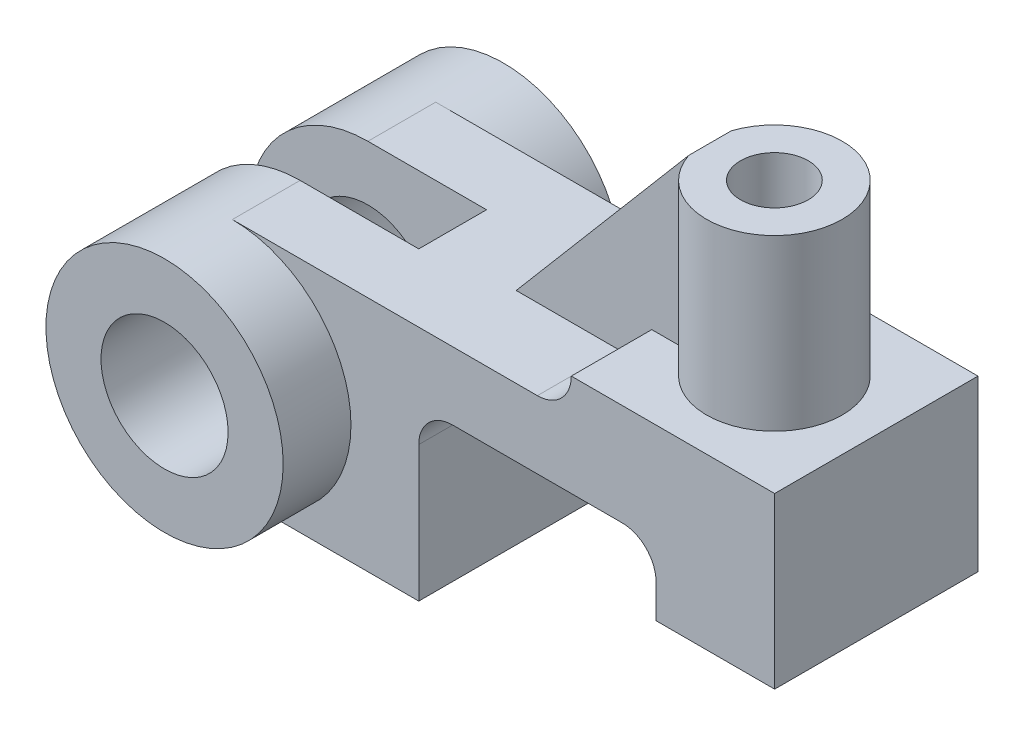
ISO-10303-21;
HEADER;
FILE_DESCRIPTION(('STEP AP214'),'2;1');
FILE_NAME('part.step','',(''),(''),'','','');
FILE_SCHEMA(('AUTOMOTIVE_DESIGN { 1 0 10303 214 1 1 1 1 }'));
ENDSEC;
DATA;
#1=APPLICATION_CONTEXT('core data for automotive mechanical design processes');
#2=APPLICATION_PROTOCOL_DEFINITION('international standard','automotive_design',2000,#1);
#3=PRODUCT_CONTEXT('',#1,'mechanical');
#4=PRODUCT('Part','Part','',(#3));
#5=PRODUCT_RELATED_PRODUCT_CATEGORY('part','',(#4));
#6=PRODUCT_DEFINITION_FORMATION('','',#4);
#7=PRODUCT_DEFINITION_CONTEXT('part definition',#1,'design');
#8=PRODUCT_DEFINITION('design','',#6,#7);
#9=PRODUCT_DEFINITION_SHAPE('','',#8);
#10=(LENGTH_UNIT() NAMED_UNIT(*) SI_UNIT(.MILLI.,.METRE.));
#11=(NAMED_UNIT(*) PLANE_ANGLE_UNIT() SI_UNIT($,.RADIAN.));
#12=(NAMED_UNIT(*) SI_UNIT($,.STERADIAN.) SOLID_ANGLE_UNIT());
#13=UNCERTAINTY_MEASURE_WITH_UNIT(LENGTH_MEASURE(1.E-05),#10,'distance_accuracy_value','');
#14=(GEOMETRIC_REPRESENTATION_CONTEXT(3) GLOBAL_UNCERTAINTY_ASSIGNED_CONTEXT((#13)) GLOBAL_UNIT_ASSIGNED_CONTEXT((#10,
#11,#12)) REPRESENTATION_CONTEXT('',''));
#15=CARTESIAN_POINT('',(0.,0.,0.));
#16=DIRECTION('',(0.,0.,1.));
#17=DIRECTION('',(1.,0.,0.));
#18=AXIS2_PLACEMENT_3D('',#15,#16,#17);
#19=CARTESIAN_POINT('',(72.,36.,24.));
#20=DIRECTION('',(0.,0.,-1.));
#21=DIRECTION('',(-1.,0.,0.));
#22=AXIS2_PLACEMENT_3D('',#19,#20,#21);
#23=CYLINDRICAL_SURFACE('',#22,8.00000000000003);
#24=DIRECTION('',(0.,0.,-1.));
#25=VECTOR('',#24,1.);
#26=CARTESIAN_POINT('',(72.,28.,24.));
#27=LINE('',#26,#25);
#28=CARTESIAN_POINT('',(72.,28.,-5.));
#29=VERTEX_POINT('',#28);
#30=CARTESIAN_POINT('',(72.,28.,-24.));
#31=VERTEX_POINT('',#30);
#32=EDGE_CURVE('E313',#29,#31,#27,.T.);
#33=ORIENTED_EDGE('',*,*,#32,.F.);
#34=CARTESIAN_POINT('',(72.,36.,-5.));
#35=DIRECTION('',(0.,0.,-1.));
#36=DIRECTION('',(-1.,0.,0.));
#37=AXIS2_PLACEMENT_3D('',#34,#35,#36);
#38=CIRCLE('',#37,8.00000000000003);
#39=CARTESIAN_POINT('',(80.,36.,-5.));
#40=VERTEX_POINT('',#39);
#41=EDGE_CURVE('E521',#40,#29,#38,.T.);
#42=ORIENTED_EDGE('',*,*,#41,.F.);
#43=DIRECTION('',(0.,0.,-1.));
#44=VECTOR('',#43,1.);
#45=CARTESIAN_POINT('',(80.,36.,24.));
#46=LINE('',#45,#44);
#47=CARTESIAN_POINT('',(80.,36.,-24.));
#48=VERTEX_POINT('',#47);
#49=EDGE_CURVE('E312',#40,#48,#46,.T.);
#50=ORIENTED_EDGE('',*,*,#49,.T.);
#51=CARTESIAN_POINT('',(72.,36.,-24.));
#52=DIRECTION('',(0.,0.,-1.));
#53=DIRECTION('',(1.,0.,0.));
#54=AXIS2_PLACEMENT_3D('',#51,#52,#53);
#55=CIRCLE('',#54,8.00000000000003);
#56=EDGE_CURVE('E304',#48,#31,#55,.T.);
#57=ORIENTED_EDGE('',*,*,#56,.T.);
#58=EDGE_LOOP('',(#33,#42,#50,#57));
#59=FACE_BOUND('',#58,.T.);
#60=ADVANCED_FACE('F44',(#59),#23,.F.);
#61=CARTESIAN_POINT('',(0.,0.,40.));
#62=DIRECTION('',(0.,0.,-1.));
#63=DIRECTION('',(-1.,0.,0.));
#64=AXIS2_PLACEMENT_3D('',#61,#62,#63);
#65=CYLINDRICAL_SURFACE('',#64,28.);
#66=CARTESIAN_POINT('',(0.,0.,-40.));
#67=DIRECTION('',(0.,0.,1.));
#68=DIRECTION('',(1.,0.,0.));
#69=AXIS2_PLACEMENT_3D('',#66,#67,#68);
#70=CIRCLE('',#69,28.);
#71=CARTESIAN_POINT('',(28.,0.,-40.));
#72=VERTEX_POINT('',#71);
#73=EDGE_CURVE('E349',#72,#72,#70,.T.);
#74=ORIENTED_EDGE('',*,*,#73,.T.);
#75=EDGE_LOOP('',(#74));
#76=FACE_BOUND('',#75,.T.);
#77=DIRECTION('',(0.,0.,-1.));
#78=VECTOR('',#77,1.);
#79=CARTESIAN_POINT('',(0.,-28.,24.));
#80=LINE('',#79,#78);
#81=CARTESIAN_POINT('',(0.,-28.,-8.));
#82=VERTEX_POINT('',#81);
#83=CARTESIAN_POINT('',(0.,-28.,-24.));
#84=VERTEX_POINT('',#83);
#85=EDGE_CURVE('E344',#82,#84,#80,.T.);
#86=ORIENTED_EDGE('',*,*,#85,.F.);
#87=CARTESIAN_POINT('',(0.,0.,-8.));
#88=DIRECTION('',(0.,0.,-1.));
#89=DIRECTION('',(-1.,0.,0.));
#90=AXIS2_PLACEMENT_3D('',#87,#88,#89);
#91=CIRCLE('',#90,28.);
#92=CARTESIAN_POINT('',(0.,28.,-8.));
#93=VERTEX_POINT('',#92);
#94=EDGE_CURVE('E250',#82,#93,#91,.T.);
#95=ORIENTED_EDGE('',*,*,#94,.T.);
#96=DIRECTION('',(0.,0.,-1.));
#97=VECTOR('',#96,1.);
#98=CARTESIAN_POINT('',(0.,28.,24.));
#99=LINE('',#98,#97);
#100=CARTESIAN_POINT('',(0.,28.,-24.));
#101=VERTEX_POINT('',#100);
#102=EDGE_CURVE('E282',#93,#101,#99,.T.);
#103=ORIENTED_EDGE('',*,*,#102,.T.);
#104=CARTESIAN_POINT('',(0.,0.,-24.));
#105=DIRECTION('',(0.,0.,-1.));
#106=DIRECTION('',(1.,0.,0.));
#107=AXIS2_PLACEMENT_3D('',#104,#105,#106);
#108=CIRCLE('',#107,28.);
#109=EDGE_CURVE('E251',#101,#84,#108,.T.);
#110=ORIENTED_EDGE('',*,*,#109,.T.);
#111=EDGE_LOOP('',(#86,#95,#103,#110));
#112=FACE_BOUND('',#111,.T.);
#113=ADVANCED_FACE('F404',(#76,#112),#65,.T.);
#114=CARTESIAN_POINT('',(0.,0.,40.));
#115=DIRECTION('',(0.,0.,-1.));
#116=DIRECTION('',(-1.,0.,0.));
#117=AXIS2_PLACEMENT_3D('',#114,#115,#116);
#118=CYLINDRICAL_SURFACE('',#117,15.);
#119=CARTESIAN_POINT('',(0.,0.,-8.));
#120=DIRECTION('',(0.,0.,-1.));
#121=DIRECTION('',(-1.,0.,0.));
#122=AXIS2_PLACEMENT_3D('',#119,#120,#121);
#123=CIRCLE('',#122,15.);
#124=CARTESIAN_POINT('',(-15.,0.,-8.));
#125=VERTEX_POINT('',#124);
#126=EDGE_CURVE('E247',#125,#125,#123,.T.);
#127=ORIENTED_EDGE('',*,*,#126,.F.);
#128=EDGE_LOOP('',(#127));
#129=FACE_BOUND('',#128,.T.);
#130=CARTESIAN_POINT('',(0.,0.,-40.));
#131=DIRECTION('',(0.,0.,1.));
#132=DIRECTION('',(1.,0.,0.));
#133=AXIS2_PLACEMENT_3D('',#130,#131,#132);
#134=CIRCLE('',#133,15.);
#135=CARTESIAN_POINT('',(15.,0.,-40.));
#136=VERTEX_POINT('',#135);
#137=EDGE_CURVE('E345',#136,#136,#134,.T.);
#138=ORIENTED_EDGE('',*,*,#137,.F.);
#139=EDGE_LOOP('',(#138));
#140=FACE_BOUND('',#139,.T.);
#141=ADVANCED_FACE('F411',(#129,#140),#118,.F.);
#142=CARTESIAN_POINT('',(0.,0.,40.));
#143=DIRECTION('',(0.,0.,1.));
#144=DIRECTION('',(1.,0.,0.));
#145=AXIS2_PLACEMENT_3D('',#142,#143,#144);
#146=PLANE('',#145);
#147=CARTESIAN_POINT('',(0.,0.,40.));
#148=DIRECTION('',(0.,0.,1.));
#149=DIRECTION('',(1.,0.,0.));
#150=AXIS2_PLACEMENT_3D('',#147,#148,#149);
#151=CIRCLE('',#150,28.);
#152=CARTESIAN_POINT('',(28.,0.,40.));
#153=VERTEX_POINT('',#152);
#154=EDGE_CURVE('E355',#153,#153,#151,.T.);
#155=ORIENTED_EDGE('',*,*,#154,.T.);
#156=EDGE_LOOP('',(#155));
#157=FACE_BOUND('',#156,.T.);
#158=CARTESIAN_POINT('',(0.,0.,40.));
#159=DIRECTION('',(0.,0.,1.));
#160=DIRECTION('',(1.,0.,0.));
#161=AXIS2_PLACEMENT_3D('',#158,#159,#160);
#162=CIRCLE('',#161,15.);
#163=CARTESIAN_POINT('',(15.,0.,40.));
#164=VERTEX_POINT('',#163);
#165=EDGE_CURVE('E347',#164,#164,#162,.T.);
#166=ORIENTED_EDGE('',*,*,#165,.F.);
#167=EDGE_LOOP('',(#166));
#168=FACE_BOUND('',#167,.T.);
#169=ADVANCED_FACE('F458',(#157,#168),#146,.T.);
#170=CARTESIAN_POINT('',(0.,0.,-40.));
#171=DIRECTION('',(0.,0.,1.));
#172=DIRECTION('',(1.,0.,0.));
#173=AXIS2_PLACEMENT_3D('',#170,#171,#172);
#174=PLANE('',#173);
#175=ORIENTED_EDGE('',*,*,#73,.F.);
#176=EDGE_LOOP('',(#175));
#177=FACE_BOUND('',#176,.T.);
#178=ORIENTED_EDGE('',*,*,#137,.T.);
#179=EDGE_LOOP('',(#178));
#180=FACE_BOUND('',#179,.T.);
#181=ADVANCED_FACE('F465',(#177,#180),#174,.F.);
#182=CARTESIAN_POINT('',(0.,28.,24.));
#183=VERTEX_POINT('',#182);
#184=CARTESIAN_POINT('',(0.,28.,8.));
#185=VERTEX_POINT('',#184);
#186=EDGE_CURVE('E306',#183,#185,#99,.T.);
#187=ORIENTED_EDGE('',*,*,#186,.T.);
#188=CARTESIAN_POINT('',(0.,0.,8.));
#189=DIRECTION('',(0.,0.,1.));
#190=DIRECTION('',(1.,0.,0.));
#191=AXIS2_PLACEMENT_3D('',#188,#189,#190);
#192=CIRCLE('',#191,28.);
#193=CARTESIAN_POINT('',(0.,-28.,8.));
#194=VERTEX_POINT('',#193);
#195=EDGE_CURVE('E58',#185,#194,#192,.T.);
#196=ORIENTED_EDGE('',*,*,#195,.T.);
#197=CARTESIAN_POINT('',(0.,-28.,24.));
#198=VERTEX_POINT('',#197);
#199=EDGE_CURVE('E67',#198,#194,#80,.T.);
#200=ORIENTED_EDGE('',*,*,#199,.F.);
#201=CARTESIAN_POINT('',(0.,0.,24.));
#202=DIRECTION('',(0.,0.,-1.));
#203=DIRECTION('',(1.,0.,0.));
#204=AXIS2_PLACEMENT_3D('',#201,#202,#203);
#205=CIRCLE('',#204,28.);
#206=EDGE_CURVE('E255',#183,#198,#205,.T.);
#207=ORIENTED_EDGE('',*,*,#206,.F.);
#208=EDGE_LOOP('',(#187,#196,#200,#207));
#209=FACE_BOUND('',#208,.T.);
#210=ORIENTED_EDGE('',*,*,#154,.F.);
#211=EDGE_LOOP('',(#210));
#212=FACE_BOUND('',#211,.T.);
#213=ADVANCED_FACE('F50',(#209,#212),#65,.T.);
#214=CARTESIAN_POINT('',(0.,0.,8.));
#215=DIRECTION('',(0.,0.,1.));
#216=DIRECTION('',(1.,0.,0.));
#217=AXIS2_PLACEMENT_3D('',#214,#215,#216);
#218=CIRCLE('',#217,15.);
#219=CARTESIAN_POINT('',(15.,0.,8.));
#220=VERTEX_POINT('',#219);
#221=EDGE_CURVE('E242',#220,#220,#218,.T.);
#222=ORIENTED_EDGE('',*,*,#221,.F.);
#223=EDGE_LOOP('',(#222));
#224=FACE_BOUND('',#223,.T.);
#225=ORIENTED_EDGE('',*,*,#165,.T.);
#226=EDGE_LOOP('',(#225));
#227=FACE_BOUND('',#226,.T.);
#228=ADVANCED_FACE('F455',(#224,#227),#118,.F.);
#229=CARTESIAN_POINT('',(44.,-28.,24.));
#230=DIRECTION('',(0.,1.,0.));
#231=DIRECTION('',(-1.,0.,0.));
#232=AXIS2_PLACEMENT_3D('',#229,#230,#231);
#233=PLANE('',#232);
#234=DIRECTION('',(0.,0.,-1.));
#235=VECTOR('',#234,1.);
#236=CARTESIAN_POINT('',(28.,-28.,-8.));
#237=LINE('',#236,#235);
#238=CARTESIAN_POINT('',(28.,-28.,8.));
#239=VERTEX_POINT('',#238);
#240=CARTESIAN_POINT('',(28.,-28.,-8.));
#241=VERTEX_POINT('',#240);
#242=EDGE_CURVE('E231',#239,#241,#237,.T.);
#243=ORIENTED_EDGE('',*,*,#242,.T.);
#244=DIRECTION('',(-1.,0.,0.));
#245=VECTOR('',#244,1.);
#246=CARTESIAN_POINT('',(-35.2475217836103,-28.,-8.));
#247=LINE('',#246,#245);
#248=EDGE_CURVE('E233',#241,#82,#247,.T.);
#249=ORIENTED_EDGE('',*,*,#248,.T.);
#250=ORIENTED_EDGE('',*,*,#85,.T.);
#251=DIRECTION('',(1.,0.,0.));
#252=VECTOR('',#251,1.);
#253=CARTESIAN_POINT('',(44.,-28.,-24.));
#254=LINE('',#253,#252);
#255=CARTESIAN_POINT('',(44.,-28.,-24.));
#256=VERTEX_POINT('',#255);
#257=EDGE_CURVE('E284',#84,#256,#254,.T.);
#258=ORIENTED_EDGE('',*,*,#257,.T.);
#259=DIRECTION('',(0.,0.,-1.));
#260=VECTOR('',#259,1.);
#261=CARTESIAN_POINT('',(44.,-28.,24.));
#262=LINE('',#261,#260);
#263=CARTESIAN_POINT('',(44.,-28.,24.));
#264=VERTEX_POINT('',#263);
#265=EDGE_CURVE('E336',#264,#256,#262,.T.);
#266=ORIENTED_EDGE('',*,*,#265,.F.);
#267=DIRECTION('',(1.,0.,0.));
#268=VECTOR('',#267,1.);
#269=CARTESIAN_POINT('',(44.,-28.,24.));
#270=LINE('',#269,#268);
#271=EDGE_CURVE('E260',#198,#264,#270,.T.);
#272=ORIENTED_EDGE('',*,*,#271,.F.);
#273=ORIENTED_EDGE('',*,*,#199,.T.);
#274=DIRECTION('',(1.,0.,0.));
#275=VECTOR('',#274,1.);
#276=CARTESIAN_POINT('',(-35.2475217836103,-28.,8.));
#277=LINE('',#276,#275);
#278=EDGE_CURVE('E228',#194,#239,#277,.T.);
#279=ORIENTED_EDGE('',*,*,#278,.T.);
#280=EDGE_LOOP('',(#243,#249,#250,#258,#266,#272,#273,#279));
#281=FACE_BOUND('',#280,.T.);
#282=ADVANCED_FACE('F451',(#281),#233,.F.);
#283=CARTESIAN_POINT('',(44.,3.99999999999999,24.));
#284=DIRECTION('',(-1.,0.,0.));
#285=DIRECTION('',(0.,0.,1.));
#286=AXIS2_PLACEMENT_3D('',#283,#284,#285);
#287=PLANE('',#286);
#288=DIRECTION('',(0.,1.,0.));
#289=VECTOR('',#288,1.);
#290=CARTESIAN_POINT('',(44.,3.99999999999999,-24.));
#291=LINE('',#290,#289);
#292=CARTESIAN_POINT('',(44.,4.,-24.));
#293=VERTEX_POINT('',#292);
#294=EDGE_CURVE('E286',#256,#293,#291,.T.);
#295=ORIENTED_EDGE('',*,*,#294,.T.);
#296=DIRECTION('',(0.,0.,-1.));
#297=VECTOR('',#296,1.);
#298=CARTESIAN_POINT('',(44.,4.,24.));
#299=LINE('',#298,#297);
#300=CARTESIAN_POINT('',(44.,4.,24.));
#301=VERTEX_POINT('',#300);
#302=EDGE_CURVE('E340',#301,#293,#299,.T.);
#303=ORIENTED_EDGE('',*,*,#302,.F.);
#304=DIRECTION('',(0.,1.,0.));
#305=VECTOR('',#304,1.);
#306=CARTESIAN_POINT('',(44.,3.99999999999999,24.));
#307=LINE('',#306,#305);
#308=EDGE_CURVE('E257',#264,#301,#307,.T.);
#309=ORIENTED_EDGE('',*,*,#308,.F.);
#310=ORIENTED_EDGE('',*,*,#265,.T.);
#311=EDGE_LOOP('',(#295,#303,#309,#310));
#312=FACE_BOUND('',#311,.T.);
#313=ADVANCED_FACE('F450',(#312),#287,.F.);
#314=CARTESIAN_POINT('',(52.,3.99999999999999,24.));
#315=DIRECTION('',(0.,0.,-1.));
#316=DIRECTION('',(-1.,0.,0.));
#317=AXIS2_PLACEMENT_3D('',#314,#315,#316);
#318=CYLINDRICAL_SURFACE('',#317,8.);
#319=CARTESIAN_POINT('',(52.,3.99999999999999,-24.));
#320=DIRECTION('',(0.,0.,-1.));
#321=DIRECTION('',(1.,0.,0.));
#322=AXIS2_PLACEMENT_3D('',#319,#320,#321);
#323=CIRCLE('',#322,8.);
#324=CARTESIAN_POINT('',(52.,12.,-24.));
#325=VERTEX_POINT('',#324);
#326=EDGE_CURVE('E289',#293,#325,#323,.T.);
#327=ORIENTED_EDGE('',*,*,#326,.T.);
#328=DIRECTION('',(0.,0.,-1.));
#329=VECTOR('',#328,1.);
#330=CARTESIAN_POINT('',(52.,12.,24.));
#331=LINE('',#330,#329);
#332=CARTESIAN_POINT('',(52.,12.,24.));
#333=VERTEX_POINT('',#332);
#334=EDGE_CURVE('E331',#333,#325,#331,.T.);
#335=ORIENTED_EDGE('',*,*,#334,.F.);
#336=CARTESIAN_POINT('',(52.,3.99999999999999,24.));
#337=DIRECTION('',(0.,0.,-1.));
#338=DIRECTION('',(1.,0.,0.));
#339=AXIS2_PLACEMENT_3D('',#336,#337,#338);
#340=CIRCLE('',#339,8.);
#341=EDGE_CURVE('E265',#301,#333,#340,.T.);
#342=ORIENTED_EDGE('',*,*,#341,.F.);
#343=ORIENTED_EDGE('',*,*,#302,.T.);
#344=EDGE_LOOP('',(#327,#335,#342,#343));
#345=FACE_BOUND('',#344,.T.);
#346=ADVANCED_FACE('F444',(#345),#318,.F.);
#347=CARTESIAN_POINT('',(92.,12.,24.));
#348=DIRECTION('',(0.,1.,0.));
#349=DIRECTION('',(-1.,0.,0.));
#350=AXIS2_PLACEMENT_3D('',#347,#348,#349);
#351=PLANE('',#350);
#352=DIRECTION('',(1.,0.,0.));
#353=VECTOR('',#352,1.);
#354=CARTESIAN_POINT('',(92.,12.,-24.));
#355=LINE('',#354,#353);
#356=CARTESIAN_POINT('',(92.,12.,-24.));
#357=VERTEX_POINT('',#356);
#358=EDGE_CURVE('E290',#325,#357,#355,.T.);
#359=ORIENTED_EDGE('',*,*,#358,.T.);
#360=DIRECTION('',(0.,0.,-1.));
#361=VECTOR('',#360,1.);
#362=CARTESIAN_POINT('',(92.,12.,24.));
#363=LINE('',#362,#361);
#364=CARTESIAN_POINT('',(92.,12.,24.));
#365=VERTEX_POINT('',#364);
#366=EDGE_CURVE('E332',#365,#357,#363,.T.);
#367=ORIENTED_EDGE('',*,*,#366,.F.);
#368=DIRECTION('',(1.,0.,0.));
#369=VECTOR('',#368,1.);
#370=CARTESIAN_POINT('',(92.,12.,24.));
#371=LINE('',#370,#369);
#372=EDGE_CURVE('E262',#333,#365,#371,.T.);
#373=ORIENTED_EDGE('',*,*,#372,.F.);
#374=ORIENTED_EDGE('',*,*,#334,.T.);
#375=EDGE_LOOP('',(#359,#367,#373,#374));
#376=FACE_BOUND('',#375,.T.);
#377=ADVANCED_FACE('F438',(#376),#351,.F.);
#378=CARTESIAN_POINT('',(92.,4.,24.));
#379=DIRECTION('',(0.,0.,-1.));
#380=DIRECTION('',(-1.,0.,0.));
#381=AXIS2_PLACEMENT_3D('',#378,#379,#380);
#382=CYLINDRICAL_SURFACE('',#381,8.);
#383=CARTESIAN_POINT('',(92.,4.,-24.));
#384=DIRECTION('',(0.,0.,-1.));
#385=DIRECTION('',(1.,0.,0.));
#386=AXIS2_PLACEMENT_3D('',#383,#384,#385);
#387=CIRCLE('',#386,8.);
#388=CARTESIAN_POINT('',(100.,4.,-24.));
#389=VERTEX_POINT('',#388);
#390=EDGE_CURVE('E295',#357,#389,#387,.T.);
#391=ORIENTED_EDGE('',*,*,#390,.T.);
#392=DIRECTION('',(0.,0.,-1.));
#393=VECTOR('',#392,1.);
#394=CARTESIAN_POINT('',(100.,4.,24.));
#395=LINE('',#394,#393);
#396=CARTESIAN_POINT('',(100.,4.,24.));
#397=VERTEX_POINT('',#396);
#398=EDGE_CURVE('E327',#397,#389,#395,.T.);
#399=ORIENTED_EDGE('',*,*,#398,.F.);
#400=CARTESIAN_POINT('',(92.,4.,24.));
#401=DIRECTION('',(0.,0.,-1.));
#402=DIRECTION('',(1.,0.,0.));
#403=AXIS2_PLACEMENT_3D('',#400,#401,#402);
#404=CIRCLE('',#403,8.);
#405=EDGE_CURVE('E266',#365,#397,#404,.T.);
#406=ORIENTED_EDGE('',*,*,#405,.F.);
#407=ORIENTED_EDGE('',*,*,#366,.T.);
#408=EDGE_LOOP('',(#391,#399,#406,#407));
#409=FACE_BOUND('',#408,.T.);
#410=ADVANCED_FACE('F434',(#409),#382,.F.);
#411=CARTESIAN_POINT('',(100.,-3.99999999999999,24.));
#412=DIRECTION('',(1.,0.,0.));
#413=DIRECTION('',(0.,0.,-1.));
#414=AXIS2_PLACEMENT_3D('',#411,#412,#413);
#415=PLANE('',#414);
#416=DIRECTION('',(0.,-1.,0.));
#417=VECTOR('',#416,1.);
#418=CARTESIAN_POINT('',(100.,-3.99999999999999,-24.));
#419=LINE('',#418,#417);
#420=CARTESIAN_POINT('',(100.,-3.99999999999999,-24.));
#421=VERTEX_POINT('',#420);
#422=EDGE_CURVE('E294',#389,#421,#419,.T.);
#423=ORIENTED_EDGE('',*,*,#422,.T.);
#424=DIRECTION('',(0.,0.,-1.));
#425=VECTOR('',#424,1.);
#426=CARTESIAN_POINT('',(100.,-3.99999999999999,24.));
#427=LINE('',#426,#425);
#428=CARTESIAN_POINT('',(100.,-3.99999999999999,24.));
#429=VERTEX_POINT('',#428);
#430=EDGE_CURVE('E324',#429,#421,#427,.T.);
#431=ORIENTED_EDGE('',*,*,#430,.F.);
#432=DIRECTION('',(0.,-1.,0.));
#433=VECTOR('',#432,1.);
#434=CARTESIAN_POINT('',(100.,-3.99999999999999,24.));
#435=LINE('',#434,#433);
#436=EDGE_CURVE('E268',#397,#429,#435,.T.);
#437=ORIENTED_EDGE('',*,*,#436,.F.);
#438=ORIENTED_EDGE('',*,*,#398,.T.);
#439=EDGE_LOOP('',(#423,#431,#437,#438));
#440=FACE_BOUND('',#439,.T.);
#441=ADVANCED_FACE('F431',(#440),#415,.F.);
#442=CARTESIAN_POINT('',(128.,-3.99999999999998,24.));
#443=DIRECTION('',(0.,1.,0.));
#444=DIRECTION('',(-1.,0.,0.));
#445=AXIS2_PLACEMENT_3D('',#442,#443,#444);
#446=PLANE('',#445);
#447=DIRECTION('',(1.,0.,0.));
#448=VECTOR('',#447,1.);
#449=CARTESIAN_POINT('',(128.,-3.99999999999998,-24.));
#450=LINE('',#449,#448);
#451=CARTESIAN_POINT('',(128.,-3.99999999999998,-24.));
#452=VERTEX_POINT('',#451);
#453=EDGE_CURVE('E297',#421,#452,#450,.T.);
#454=ORIENTED_EDGE('',*,*,#453,.T.);
#455=DIRECTION('',(0.,0.,-1.));
#456=VECTOR('',#455,1.);
#457=CARTESIAN_POINT('',(128.,-3.99999999999998,24.));
#458=LINE('',#457,#456);
#459=CARTESIAN_POINT('',(128.,-3.99999999999998,24.));
#460=VERTEX_POINT('',#459);
#461=EDGE_CURVE('E325',#460,#452,#458,.T.);
#462=ORIENTED_EDGE('',*,*,#461,.F.);
#463=DIRECTION('',(1.,0.,0.));
#464=VECTOR('',#463,1.);
#465=CARTESIAN_POINT('',(128.,-3.99999999999998,24.));
#466=LINE('',#465,#464);
#467=EDGE_CURVE('E269',#429,#460,#466,.T.);
#468=ORIENTED_EDGE('',*,*,#467,.F.);
#469=ORIENTED_EDGE('',*,*,#430,.T.);
#470=EDGE_LOOP('',(#454,#462,#468,#469));
#471=FACE_BOUND('',#470,.T.);
#472=ADVANCED_FACE('F424',(#471),#446,.F.);
#473=CARTESIAN_POINT('',(128.,36.,24.));
#474=DIRECTION('',(-1.,0.,0.));
#475=DIRECTION('',(0.,0.,1.));
#476=AXIS2_PLACEMENT_3D('',#473,#474,#475);
#477=PLANE('',#476);
#478=DIRECTION('',(0.,1.,0.));
#479=VECTOR('',#478,1.);
#480=CARTESIAN_POINT('',(128.,36.,-24.));
#481=LINE('',#480,#479);
#482=CARTESIAN_POINT('',(128.,36.,-24.));
#483=VERTEX_POINT('',#482);
#484=EDGE_CURVE('E298',#452,#483,#481,.T.);
#485=ORIENTED_EDGE('',*,*,#484,.T.);
#486=DIRECTION('',(0.,0.,-1.));
#487=VECTOR('',#486,1.);
#488=CARTESIAN_POINT('',(128.,36.,24.));
#489=LINE('',#488,#487);
#490=CARTESIAN_POINT('',(128.,36.,24.));
#491=VERTEX_POINT('',#490);
#492=EDGE_CURVE('E317',#491,#483,#489,.T.);
#493=ORIENTED_EDGE('',*,*,#492,.F.);
#494=DIRECTION('',(0.,1.,0.));
#495=VECTOR('',#494,1.);
#496=CARTESIAN_POINT('',(128.,36.,24.));
#497=LINE('',#496,#495);
#498=EDGE_CURVE('E275',#460,#491,#497,.T.);
#499=ORIENTED_EDGE('',*,*,#498,.F.);
#500=ORIENTED_EDGE('',*,*,#461,.T.);
#501=EDGE_LOOP('',(#485,#493,#499,#500));
#502=FACE_BOUND('',#501,.T.);
#503=ADVANCED_FACE('F420',(#502),#477,.F.);
#504=CARTESIAN_POINT('',(80.,36.,24.));
#505=DIRECTION('',(0.,-1.,0.));
#506=DIRECTION('',(1.,0.,0.));
#507=AXIS2_PLACEMENT_3D('',#504,#505,#506);
#508=PLANE('',#507);
#509=ORIENTED_EDGE('',*,*,#49,.F.);
#510=DIRECTION('',(-1.,0.,0.));
#511=VECTOR('',#510,1.);
#512=CARTESIAN_POINT('',(48.,36.,-5.));
#513=LINE('',#512,#511);
#514=CARTESIAN_POINT('',(88.7437259780129,36.,-5.));
#515=VERTEX_POINT('',#514);
#516=EDGE_CURVE('E519',#515,#40,#513,.T.);
#517=ORIENTED_EDGE('',*,*,#516,.F.);
#518=CARTESIAN_POINT('',(103.942410131584,36.,0.));
#519=DIRECTION('',(0.,-1.,0.));
#520=DIRECTION('',(1.,0.,0.));
#521=AXIS2_PLACEMENT_3D('',#518,#519,#520);
#522=CIRCLE('',#521,16.);
#523=CARTESIAN_POINT('',(88.7437259780129,36.,5.));
#524=VERTEX_POINT('',#523);
#525=EDGE_CURVE('E11',#524,#515,#522,.F.);
#526=ORIENTED_EDGE('',*,*,#525,.F.);
#527=DIRECTION('',(1.,0.,0.));
#528=VECTOR('',#527,1.);
#529=CARTESIAN_POINT('',(48.,36.,5.));
#530=LINE('',#529,#528);
#531=CARTESIAN_POINT('',(80.,36.,5.));
#532=VERTEX_POINT('',#531);
#533=EDGE_CURVE('E376',#532,#524,#530,.T.);
#534=ORIENTED_EDGE('',*,*,#533,.F.);
#535=CARTESIAN_POINT('',(80.,36.,24.));
#536=VERTEX_POINT('',#535);
#537=EDGE_CURVE('E316',#536,#532,#46,.T.);
#538=ORIENTED_EDGE('',*,*,#537,.F.);
#539=DIRECTION('',(-1.,0.,0.));
#540=VECTOR('',#539,1.);
#541=CARTESIAN_POINT('',(80.,36.,24.));
#542=LINE('',#541,#540);
#543=EDGE_CURVE('E273',#491,#536,#542,.T.);
#544=ORIENTED_EDGE('',*,*,#543,.F.);
#545=ORIENTED_EDGE('',*,*,#492,.T.);
#546=DIRECTION('',(-1.,0.,0.));
#547=VECTOR('',#546,1.);
#548=CARTESIAN_POINT('',(80.,36.,-24.));
#549=LINE('',#548,#547);
#550=EDGE_CURVE('E296',#483,#48,#549,.T.);
#551=ORIENTED_EDGE('',*,*,#550,.T.);
#552=EDGE_LOOP('',(#509,#517,#526,#534,#538,#544,#545,#551));
#553=FACE_BOUND('',#552,.T.);
#554=ADVANCED_FACE('F397',(#553),#508,.F.);
#555=ORIENTED_EDGE('',*,*,#537,.T.);
#556=CARTESIAN_POINT('',(72.,36.,5.));
#557=DIRECTION('',(0.,0.,1.));
#558=DIRECTION('',(1.,0.,0.));
#559=AXIS2_PLACEMENT_3D('',#556,#557,#558);
#560=CIRCLE('',#559,8.00000000000003);
#561=CARTESIAN_POINT('',(72.,28.,5.));
#562=VERTEX_POINT('',#561);
#563=EDGE_CURVE('E375',#562,#532,#560,.T.);
#564=ORIENTED_EDGE('',*,*,#563,.F.);
#565=CARTESIAN_POINT('',(72.,28.,24.));
#566=VERTEX_POINT('',#565);
#567=EDGE_CURVE('E315',#566,#562,#27,.T.);
#568=ORIENTED_EDGE('',*,*,#567,.F.);
#569=CARTESIAN_POINT('',(72.,36.,24.));
#570=DIRECTION('',(0.,0.,-1.));
#571=DIRECTION('',(1.,0.,0.));
#572=AXIS2_PLACEMENT_3D('',#569,#570,#571);
#573=CIRCLE('',#572,8.00000000000003);
#574=EDGE_CURVE('E277',#536,#566,#573,.T.);
#575=ORIENTED_EDGE('',*,*,#574,.F.);
#576=EDGE_LOOP('',(#555,#564,#568,#575));
#577=FACE_BOUND('',#576,.T.);
#578=ADVANCED_FACE('F371',(#577),#23,.F.);
#579=CARTESIAN_POINT('',(0.,28.,24.));
#580=DIRECTION('',(0.,-1.,0.));
#581=DIRECTION('',(0.,0.,-1.));
#582=AXIS2_PLACEMENT_3D('',#579,#580,#581);
#583=PLANE('',#582);
#584=DIRECTION('',(0.,0.,1.));
#585=VECTOR('',#584,1.);
#586=CARTESIAN_POINT('',(48.,28.,-5.));
#587=LINE('',#586,#585);
#588=CARTESIAN_POINT('',(48.,28.,-5.));
#589=VERTEX_POINT('',#588);
#590=CARTESIAN_POINT('',(48.,28.,5.));
#591=VERTEX_POINT('',#590);
#592=EDGE_CURVE('E378',#589,#591,#587,.T.);
#593=ORIENTED_EDGE('',*,*,#592,.F.);
#594=DIRECTION('',(-1.,0.,0.));
#595=VECTOR('',#594,1.);
#596=CARTESIAN_POINT('',(48.,28.,-5.));
#597=LINE('',#596,#595);
#598=EDGE_CURVE('E204',#29,#589,#597,.T.);
#599=ORIENTED_EDGE('',*,*,#598,.F.);
#600=ORIENTED_EDGE('',*,*,#32,.T.);
#601=DIRECTION('',(-1.,0.,0.));
#602=VECTOR('',#601,1.);
#603=CARTESIAN_POINT('',(0.,28.,-24.));
#604=LINE('',#603,#602);
#605=EDGE_CURVE('E256',#31,#101,#604,.T.);
#606=ORIENTED_EDGE('',*,*,#605,.T.);
#607=ORIENTED_EDGE('',*,*,#102,.F.);
#608=DIRECTION('',(-1.,0.,0.));
#609=VECTOR('',#608,1.);
#610=CARTESIAN_POINT('',(-35.2475217836103,28.,-8.));
#611=LINE('',#610,#609);
#612=CARTESIAN_POINT('',(28.,28.,-8.));
#613=VERTEX_POINT('',#612);
#614=EDGE_CURVE('E222',#613,#93,#611,.T.);
#615=ORIENTED_EDGE('',*,*,#614,.F.);
#616=DIRECTION('',(0.,0.,-1.));
#617=VECTOR('',#616,1.);
#618=CARTESIAN_POINT('',(28.,28.,-8.));
#619=LINE('',#618,#617);
#620=CARTESIAN_POINT('',(28.,28.,8.));
#621=VERTEX_POINT('',#620);
#622=EDGE_CURVE('E220',#621,#613,#619,.T.);
#623=ORIENTED_EDGE('',*,*,#622,.F.);
#624=DIRECTION('',(-1.,0.,0.));
#625=VECTOR('',#624,1.);
#626=CARTESIAN_POINT('',(0.,28.,8.));
#627=LINE('',#626,#625);
#628=EDGE_CURVE('E52',#621,#185,#627,.T.);
#629=ORIENTED_EDGE('',*,*,#628,.T.);
#630=ORIENTED_EDGE('',*,*,#186,.F.);
#631=DIRECTION('',(-1.,0.,0.));
#632=VECTOR('',#631,1.);
#633=CARTESIAN_POINT('',(0.,28.,24.));
#634=LINE('',#633,#632);
#635=EDGE_CURVE('E279',#566,#183,#634,.T.);
#636=ORIENTED_EDGE('',*,*,#635,.F.);
#637=ORIENTED_EDGE('',*,*,#567,.T.);
#638=DIRECTION('',(1.,0.,0.));
#639=VECTOR('',#638,1.);
#640=CARTESIAN_POINT('',(48.,28.,5.));
#641=LINE('',#640,#639);
#642=EDGE_CURVE('E366',#591,#562,#641,.T.);
#643=ORIENTED_EDGE('',*,*,#642,.F.);
#644=EDGE_LOOP('',(#593,#599,#600,#606,#607,#615,#623,#629,#630,#636,#637,#643));
#645=FACE_BOUND('',#644,.T.);
#646=ADVANCED_FACE('F358',(#645),#583,.F.);
#647=CARTESIAN_POINT('',(0.,0.,24.));
#648=DIRECTION('',(0.,0.,1.));
#649=DIRECTION('',(1.,0.,0.));
#650=AXIS2_PLACEMENT_3D('',#647,#648,#649);
#651=PLANE('',#650);
#652=ORIENTED_EDGE('',*,*,#206,.T.);
#653=ORIENTED_EDGE('',*,*,#271,.T.);
#654=ORIENTED_EDGE('',*,*,#308,.T.);
#655=ORIENTED_EDGE('',*,*,#341,.T.);
#656=ORIENTED_EDGE('',*,*,#372,.T.);
#657=ORIENTED_EDGE('',*,*,#405,.T.);
#658=ORIENTED_EDGE('',*,*,#436,.T.);
#659=ORIENTED_EDGE('',*,*,#467,.T.);
#660=ORIENTED_EDGE('',*,*,#498,.T.);
#661=ORIENTED_EDGE('',*,*,#543,.T.);
#662=ORIENTED_EDGE('',*,*,#574,.T.);
#663=ORIENTED_EDGE('',*,*,#635,.T.);
#664=EDGE_LOOP('',(#652,#653,#654,#655,#656,#657,#658,#659,#660,#661,#662,#663));
#665=FACE_BOUND('',#664,.T.);
#666=ADVANCED_FACE('F365',(#665),#651,.T.);
#667=CARTESIAN_POINT('',(0.,0.,-24.));
#668=DIRECTION('',(0.,0.,1.));
#669=DIRECTION('',(1.,0.,0.));
#670=AXIS2_PLACEMENT_3D('',#667,#668,#669);
#671=PLANE('',#670);
#672=ORIENTED_EDGE('',*,*,#109,.F.);
#673=ORIENTED_EDGE('',*,*,#605,.F.);
#674=ORIENTED_EDGE('',*,*,#56,.F.);
#675=ORIENTED_EDGE('',*,*,#550,.F.);
#676=ORIENTED_EDGE('',*,*,#484,.F.);
#677=ORIENTED_EDGE('',*,*,#453,.F.);
#678=ORIENTED_EDGE('',*,*,#422,.F.);
#679=ORIENTED_EDGE('',*,*,#390,.F.);
#680=ORIENTED_EDGE('',*,*,#358,.F.);
#681=ORIENTED_EDGE('',*,*,#326,.F.);
#682=ORIENTED_EDGE('',*,*,#294,.F.);
#683=ORIENTED_EDGE('',*,*,#257,.F.);
#684=EDGE_LOOP('',(#672,#673,#674,#675,#676,#677,#678,#679,#680,#681,#682,#683));
#685=FACE_BOUND('',#684,.T.);
#686=ADVANCED_FACE('F483',(#685),#671,.F.);
#687=CARTESIAN_POINT('',(-35.2475217836103,-28.,-8.));
#688=DIRECTION('',(0.,0.,-1.));
#689=DIRECTION('',(-1.,0.,0.));
#690=AXIS2_PLACEMENT_3D('',#687,#688,#689);
#691=PLANE('',#690);
#692=ORIENTED_EDGE('',*,*,#126,.T.);
#693=EDGE_LOOP('',(#692));
#694=FACE_BOUND('',#693,.T.);
#695=ORIENTED_EDGE('',*,*,#248,.F.);
#696=DIRECTION('',(0.,1.,0.));
#697=VECTOR('',#696,1.);
#698=CARTESIAN_POINT('',(28.,-28.,-8.));
#699=LINE('',#698,#697);
#700=EDGE_CURVE('E239',#241,#613,#699,.T.);
#701=ORIENTED_EDGE('',*,*,#700,.T.);
#702=ORIENTED_EDGE('',*,*,#614,.T.);
#703=ORIENTED_EDGE('',*,*,#94,.F.);
#704=EDGE_LOOP('',(#695,#701,#702,#703));
#705=FACE_BOUND('',#704,.T.);
#706=ADVANCED_FACE('F479',(#694,#705),#691,.F.);
#707=CARTESIAN_POINT('',(-35.2475217836103,-28.,8.));
#708=DIRECTION('',(0.,0.,1.));
#709=DIRECTION('',(1.,0.,0.));
#710=AXIS2_PLACEMENT_3D('',#707,#708,#709);
#711=PLANE('',#710);
#712=ORIENTED_EDGE('',*,*,#221,.T.);
#713=EDGE_LOOP('',(#712));
#714=FACE_BOUND('',#713,.T.);
#715=ORIENTED_EDGE('',*,*,#628,.F.);
#716=DIRECTION('',(0.,1.,0.));
#717=VECTOR('',#716,1.);
#718=CARTESIAN_POINT('',(28.,-28.,8.));
#719=LINE('',#718,#717);
#720=EDGE_CURVE('E237',#239,#621,#719,.T.);
#721=ORIENTED_EDGE('',*,*,#720,.F.);
#722=ORIENTED_EDGE('',*,*,#278,.F.);
#723=ORIENTED_EDGE('',*,*,#195,.F.);
#724=EDGE_LOOP('',(#715,#721,#722,#723));
#725=FACE_BOUND('',#724,.T.);
#726=ADVANCED_FACE('F485',(#714,#725),#711,.F.);
#727=CARTESIAN_POINT('',(28.,-28.,-8.));
#728=DIRECTION('',(1.,0.,0.));
#729=DIRECTION('',(0.,0.,-1.));
#730=AXIS2_PLACEMENT_3D('',#727,#728,#729);
#731=PLANE('',#730);
#732=ORIENTED_EDGE('',*,*,#622,.T.);
#733=ORIENTED_EDGE('',*,*,#700,.F.);
#734=ORIENTED_EDGE('',*,*,#242,.F.);
#735=ORIENTED_EDGE('',*,*,#720,.T.);
#736=EDGE_LOOP('',(#732,#733,#734,#735));
#737=FACE_BOUND('',#736,.T.);
#738=ADVANCED_FACE('F487',(#737),#731,.F.);
#739=CARTESIAN_POINT('',(103.942410131584,76.,0.));
#740=DIRECTION('',(0.,1.,0.));
#741=DIRECTION('',(-1.,0.,0.));
#742=AXIS2_PLACEMENT_3D('',#739,#740,#741);
#743=PLANE('',#742);
#744=DIRECTION('',(0.,0.,1.));
#745=VECTOR('',#744,1.);
#746=CARTESIAN_POINT('',(88.7437259780129,76.,-5.));
#747=LINE('',#746,#745);
#748=CARTESIAN_POINT('',(88.7437259780129,76.,-5.));
#749=VERTEX_POINT('',#748);
#750=CARTESIAN_POINT('',(88.7437259780129,76.,5.));
#751=VERTEX_POINT('',#750);
#752=EDGE_CURVE('E190',#749,#751,#747,.T.);
#753=ORIENTED_EDGE('',*,*,#752,.T.);
#754=CARTESIAN_POINT('',(103.942410131584,76.,0.));
#755=DIRECTION('',(0.,1.,0.));
#756=DIRECTION('',(-1.,0.,0.));
#757=AXIS2_PLACEMENT_3D('',#754,#755,#756);
#758=CIRCLE('',#757,16.);
#759=EDGE_CURVE('E211',#751,#749,#758,.T.);
#760=ORIENTED_EDGE('',*,*,#759,.T.);
#761=EDGE_LOOP('',(#753,#760));
#762=FACE_BOUND('',#761,.T.);
#763=CARTESIAN_POINT('',(103.942410131584,76.,0.));
#764=DIRECTION('',(0.,1.,0.));
#765=DIRECTION('',(-1.,0.,0.));
#766=AXIS2_PLACEMENT_3D('',#763,#764,#765);
#767=CIRCLE('',#766,8.00000000000001);
#768=CARTESIAN_POINT('',(95.9424101315836,76.,0.));
#769=VERTEX_POINT('',#768);
#770=EDGE_CURVE('E217',#769,#769,#767,.T.);
#771=ORIENTED_EDGE('',*,*,#770,.F.);
#772=EDGE_LOOP('',(#771));
#773=FACE_BOUND('',#772,.T.);
#774=ADVANCED_FACE('F214',(#762,#773),#743,.T.);
#775=CARTESIAN_POINT('',(103.942410131584,76.,0.));
#776=DIRECTION('',(0.,-1.,0.));
#777=DIRECTION('',(1.,0.,0.));
#778=AXIS2_PLACEMENT_3D('',#775,#776,#777);
#779=CYLINDRICAL_SURFACE('',#778,16.);
#780=ORIENTED_EDGE('',*,*,#525,.T.);
#781=DIRECTION('',(0.,1.,0.));
#782=VECTOR('',#781,1.);
#783=CARTESIAN_POINT('',(88.7437259780129,-28.002,-5.));
#784=LINE('',#783,#782);
#785=EDGE_CURVE('E197',#515,#749,#784,.T.);
#786=ORIENTED_EDGE('',*,*,#785,.T.);
#787=ORIENTED_EDGE('',*,*,#759,.F.);
#788=DIRECTION('',(0.,1.,0.));
#789=VECTOR('',#788,1.);
#790=CARTESIAN_POINT('',(88.7437259780129,-28.002,5.));
#791=LINE('',#790,#789);
#792=EDGE_CURVE('E213',#524,#751,#791,.T.);
#793=ORIENTED_EDGE('',*,*,#792,.F.);
#794=EDGE_LOOP('',(#780,#786,#787,#793));
#795=FACE_BOUND('',#794,.T.);
#796=ADVANCED_FACE('F207',(#795),#779,.T.);
#797=CARTESIAN_POINT('',(103.942410131584,76.,0.));
#798=DIRECTION('',(0.,-1.,0.));
#799=DIRECTION('',(1.,0.,0.));
#800=AXIS2_PLACEMENT_3D('',#797,#798,#799);
#801=CYLINDRICAL_SURFACE('',#800,8.00000000000001);
#802=ORIENTED_EDGE('',*,*,#770,.T.);
#803=EDGE_LOOP('',(#802));
#804=FACE_BOUND('',#803,.T.);
#805=CARTESIAN_POINT('',(103.942410131584,36.,0.));
#806=DIRECTION('',(0.,1.,0.));
#807=DIRECTION('',(-1.,0.,0.));
#808=AXIS2_PLACEMENT_3D('',#805,#806,#807);
#809=CIRCLE('',#808,8.00000000000001);
#810=CARTESIAN_POINT('',(95.9424101315836,36.,0.));
#811=VERTEX_POINT('',#810);
#812=EDGE_CURVE('E221',#811,#811,#809,.T.);
#813=ORIENTED_EDGE('',*,*,#812,.F.);
#814=EDGE_LOOP('',(#813));
#815=FACE_BOUND('',#814,.T.);
#816=ADVANCED_FACE('F389',(#804,#815),#801,.F.);
#817=ORIENTED_EDGE('',*,*,#812,.T.);
#818=EDGE_LOOP('',(#817));
#819=FACE_BOUND('',#818,.T.);
#820=ADVANCED_FACE('F387',(#819),#508,.F.);
#821=CARTESIAN_POINT('',(48.,-28.002,-5.));
#822=DIRECTION('',(0.,0.,-1.));
#823=DIRECTION('',(-1.,0.,0.));
#824=AXIS2_PLACEMENT_3D('',#821,#822,#823);
#825=PLANE('',#824);
#826=DIRECTION('',(0.647129375374689,0.762380201426536,0.));
#827=VECTOR('',#826,1.);
#828=CARTESIAN_POINT('',(88.7437259780129,76.,-5.));
#829=LINE('',#828,#827);
#830=EDGE_CURVE('E186',#589,#749,#829,.T.);
#831=ORIENTED_EDGE('',*,*,#830,.T.);
#832=ORIENTED_EDGE('',*,*,#785,.F.);
#833=ORIENTED_EDGE('',*,*,#516,.T.);
#834=ORIENTED_EDGE('',*,*,#41,.T.);
#835=ORIENTED_EDGE('',*,*,#598,.T.);
#836=EDGE_LOOP('',(#831,#832,#833,#834,#835));
#837=FACE_BOUND('',#836,.T.);
#838=ADVANCED_FACE('F203',(#837),#825,.T.);
#839=CARTESIAN_POINT('',(48.,-28.002,5.));
#840=DIRECTION('',(0.,0.,1.));
#841=DIRECTION('',(1.,0.,0.));
#842=AXIS2_PLACEMENT_3D('',#839,#840,#841);
#843=PLANE('',#842);
#844=DIRECTION('',(0.647129375374689,0.762380201426536,0.));
#845=VECTOR('',#844,1.);
#846=CARTESIAN_POINT('',(88.7437259780129,76.,5.));
#847=LINE('',#846,#845);
#848=EDGE_CURVE('E194',#591,#751,#847,.T.);
#849=ORIENTED_EDGE('',*,*,#848,.F.);
#850=ORIENTED_EDGE('',*,*,#642,.T.);
#851=ORIENTED_EDGE('',*,*,#563,.T.);
#852=ORIENTED_EDGE('',*,*,#533,.T.);
#853=ORIENTED_EDGE('',*,*,#792,.T.);
#854=EDGE_LOOP('',(#849,#850,#851,#852,#853));
#855=FACE_BOUND('',#854,.T.);
#856=ADVANCED_FACE('F399',(#855),#843,.T.);
#857=CARTESIAN_POINT('',(88.7437259780129,76.,-5.));
#858=DIRECTION('',(0.762380201426536,-0.647129375374689,0.));
#859=DIRECTION('',(0.647129375374689,0.762380201426536,0.));
#860=AXIS2_PLACEMENT_3D('',#857,#858,#859);
#861=PLANE('',#860);
#862=ORIENTED_EDGE('',*,*,#848,.T.);
#863=ORIENTED_EDGE('',*,*,#752,.F.);
#864=ORIENTED_EDGE('',*,*,#830,.F.);
#865=ORIENTED_EDGE('',*,*,#592,.T.);
#866=EDGE_LOOP('',(#862,#863,#864,#865));
#867=FACE_BOUND('',#866,.T.);
#868=ADVANCED_FACE('F189',(#867),#861,.F.);
#869=CLOSED_SHELL('',(#60,#113,#141,#169,#181,#213,#228,#282,#313,#346,#377,#410,#441,#472,#503,
#554,#578,#646,#666,#686,#706,#726,#738,#774,#796,#816,#820,#838,#856,#868));
#870=MANIFOLD_SOLID_BREP('B2',#869);
#871=ADVANCED_BREP_SHAPE_REPRESENTATION('',(#18,#870),#14);
#872=SHAPE_DEFINITION_REPRESENTATION(#9,#871);
ENDSEC;
END-ISO-10303-21;
